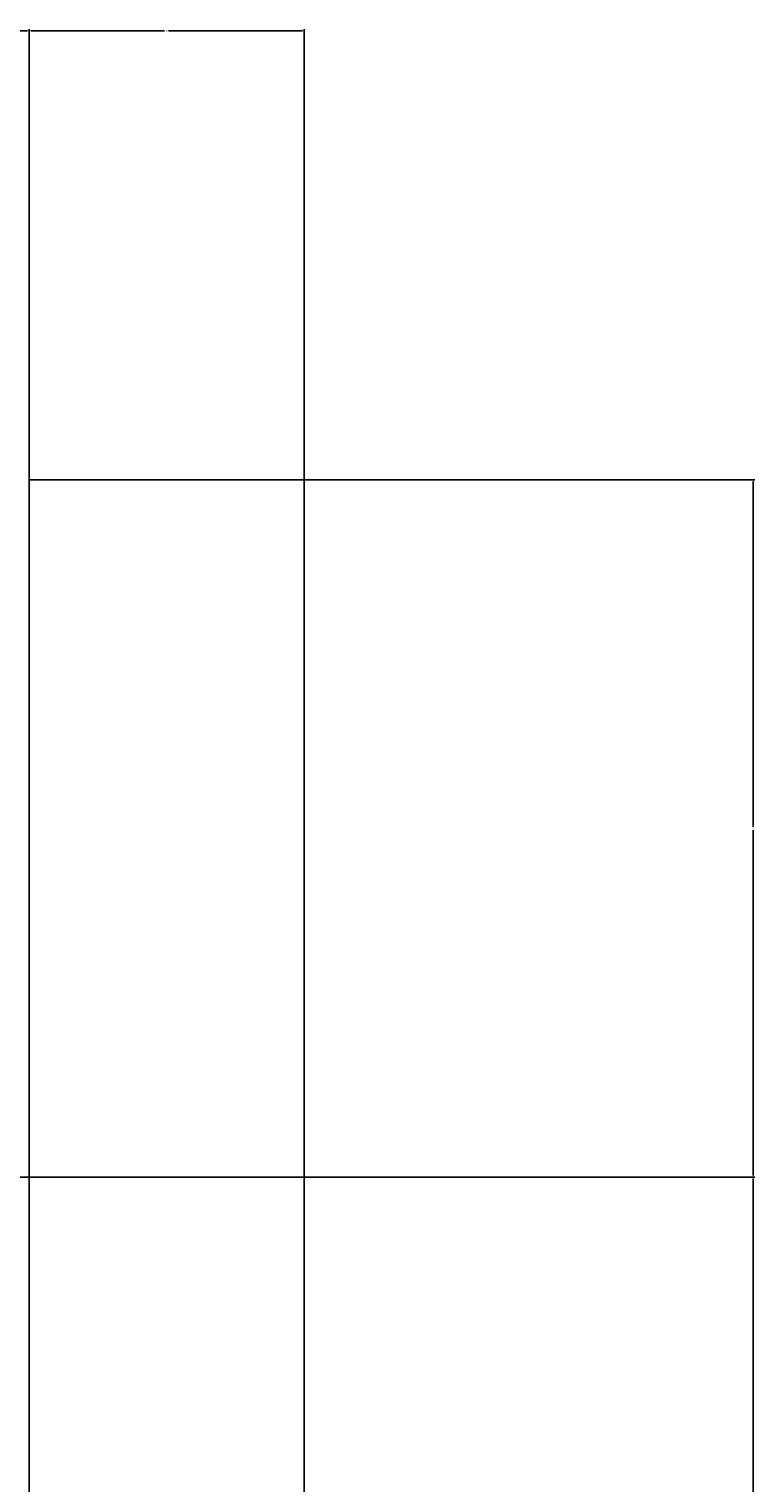
# Model space of a CAD drawing. Units: inches. Extents: x 3731 to 4318, y 1310 to 2388.
# Tile 57 of 57: x 4239 to 4318, y 2229 to 2388. Entities that reach past the tile are written whole.
import ezdxf

# ---------------------------------------------------------------- set-up
doc = ezdxf.new("R2010")
doc.units = ezdxf.units.IN
doc.layers.add('A-ANNO-DIMS', color=2, linetype='Continuous', lineweight=18)
doc.styles.get("Standard").update_dxf_attribs({"font": 'arial.ttf'})
doc.dimstyles.get("Standard").update_dxf_attribs({"dimtxt": 0.18, "dimasz": 0.18, "dimexe": 0.18, "dimexo": 0.0625, "dimgap": 0.09, "dimtad": 0, "dimtih": 1, "dimtoh": 1, "dimdec": 4, "dimzin": 0, "dimdsep": 46, "dimtxsty": 'Standard', "dimcen": 0.09, "dimadec": 0, "dimazin": 0, "dimtfac": 1, "dimtdec": 4, "dimtofl": 0, "dimtmove": 0, "dimatfit": 3, "dimfxl": 1, "dimtolj": 1, "dimtzin": 0, "dimarcsym": 0})

# ---------------------------------------------------------------- blocks, each defined once
blk = doc.blocks.new('*D36')
at = {"layer": 'A-ANNO-DIMS', "color": 0, "lineweight": -2, "transparency": 16777216}
for p, q in [((4103.21, 2338.44), (4103.21, 2387.51)), ((4103.39, 2387.33), (4170.93, 2387.33)), ((4239.03, 2387.33), (4171.49, 2387.33)), ((4239.21, 2338.44), (4239.21, 2387.51))]:
    blk.add_line(p, q, dxfattribs=at)
at = {"layer": 'A-ANNO-DIMS', "color": 0, "transparency": 16777216}
for points in [[(4103.39, 2387.36), (4103.39, 2387.3), (4103.21, 2387.33)], [(4239.03, 2387.36), (4239.03, 2387.3), (4239.21, 2387.33)]]:
    blk.add_solid(points, dxfattribs=at)
at = {"layer": 'Defpoints', "color": 0, "transparency": 16777216}
for p in [(4239.21, 2387.33), (4103.21, 2338.38), (4239.21, 2338.38)]:
    blk.add_point(p, dxfattribs=at)
at = {"layer": 'A-ANNO-DIMS', "color": 0, "transparency": 16777216, "insert": (4171.21, 2387.33), "char_height": 0.18, "attachment_point": 5}
blk.add_mtext('\\A1;136', dxfattribs=at)
blk = doc.blocks.new('*D37')
at = {"layer": 'A-ANNO-DIMS', "color": 0, "lineweight": -2, "transparency": 16777216}
for p, q in [((4239.27, 2338.38), (4318.34, 2338.38)), ((4318.16, 2338.2), (4318.16, 2300.56)), ((4318.16, 2262.56), (4318.16, 2300.2)), ((4103.27, 2262.38), (4318.34, 2262.38))]:
    blk.add_line(p, q, dxfattribs=at)
at = {"layer": 'A-ANNO-DIMS', "color": 0, "transparency": 16777216}
for points in [[(4318.13, 2338.2), (4318.19, 2338.2), (4318.16, 2338.38)], [(4318.13, 2262.56), (4318.19, 2262.56), (4318.16, 2262.38)]]:
    blk.add_solid(points, dxfattribs=at)
at = {"layer": 'Defpoints', "color": 0, "transparency": 16777216}
for p in [(4239.21, 2338.38), (4318.16, 2338.38), (4103.21, 2262.38)]:
    blk.add_point(p, dxfattribs=at)
at = {"layer": 'A-ANNO-DIMS', "color": 0, "transparency": 16777216, "insert": (4318.16, 2300.38), "char_height": 0.18, "attachment_point": 5}
blk.add_mtext('\\A1;76', dxfattribs=at)
blk = doc.blocks.new('*D38')
at = {"layer": 'A-ANNO-DIMS', "color": 0, "lineweight": -2, "transparency": 16777216}
for p, q in [((4103.27, 2262.38), (4318.34, 2262.38)), ((4318.16, 2262.2), (4318.16, 2103.06)), ((4318.16, 1943.56), (4318.16, 2102.7)), ((4234.27, 1943.38), (4318.34, 1943.38))]:
    blk.add_line(p, q, dxfattribs=at)
at = {"layer": 'A-ANNO-DIMS', "color": 0, "transparency": 16777216}
for points in [[(4318.13, 2262.2), (4318.19, 2262.2), (4318.16, 2262.38)], [(4318.13, 1943.56), (4318.19, 1943.56), (4318.16, 1943.38)]]:
    blk.add_solid(points, dxfattribs=at)
at = {"layer": 'Defpoints', "color": 0, "transparency": 16777216}
for p in [(4103.21, 2262.38), (4318.16, 2262.38), (4234.21, 1943.38)]:
    blk.add_point(p, dxfattribs=at)
at = {"layer": 'A-ANNO-DIMS', "color": 0, "transparency": 16777216, "insert": (4318.16, 2102.88), "char_height": 0.18, "attachment_point": 5}
blk.add_mtext('\\A1;319', dxfattribs=at)
blk = doc.blocks.new('*D51')
at = {"layer": 'A-ANNO-DIMS', "color": 0, "lineweight": -2, "transparency": 16777216}
for p, q in [((4239.21, 1708.44), (4239.21, 2387.51)), ((4239.39, 2387.33), (4253.99, 2387.33)), ((4269.03, 2387.33), (4254.43, 2387.33)), ((4269.21, 1708.44), (4269.21, 2387.51))]:
    blk.add_line(p, q, dxfattribs=at)
at = {"layer": 'A-ANNO-DIMS', "color": 0, "transparency": 16777216}
for points in [[(4239.39, 2387.36), (4239.39, 2387.3), (4239.21, 2387.33)], [(4269.03, 2387.36), (4269.03, 2387.3), (4269.21, 2387.33)]]:
    blk.add_solid(points, dxfattribs=at)
at = {"layer": 'Defpoints', "color": 0, "transparency": 16777216}
for p in [(4269.21, 2387.33), (4239.21, 1708.38), (4269.21, 1708.38)]:
    blk.add_point(p, dxfattribs=at)
at = {"layer": 'A-ANNO-DIMS', "color": 0, "transparency": 16777216, "insert": (4254.21, 2387.33), "char_height": 0.18, "attachment_point": 5}
blk.add_mtext('\\A1;30', dxfattribs=at)

msp = doc.modelspace()

# ---------------------------------------------------------------- dimensions: what is measured, and where the dimension line sits
at = {"layer": 'A-ANNO-DIMS'}
for base, p1, p2, picture, middle in [((4239.21, 2387.33), (4103.21, 2338.38), (4239.21, 2338.38), '*D36', (4171.21, 2387.33)), ((4269.21, 2387.33), (4239.21, 1708.38), (4269.21, 1708.38), '*D51', (4254.21, 2387.33))]:
    dim = msp.add_linear_dim(base=base, p1=p1, p2=p2, dimstyle='Standard', override={"dimdec": 0, "dimlfac": 1, "dimrnd": 0, "dimzin": 0, "dimdsep": 46, "dimlunit": 2}, dxfattribs=at)
    dim.commit()
    dim.dimension.update_dxf_attribs({"geometry": picture, "text_midpoint": middle})
for base, p1, p2, picture, middle in [((4318.16, 2338.38), (4103.21, 2262.38), (4239.21, 2338.38), '*D37', (4318.16, 2300.38)), ((4318.16, 2262.38), (4234.21, 1943.38), (4103.21, 2262.38), '*D38', (4318.16, 2102.88))]:
    dim = msp.add_linear_dim(base=base, p1=p1, p2=p2, angle=90, dimstyle='Standard', override={"dimdec": 0, "dimlfac": 1, "dimrnd": 0, "dimzin": 0, "dimdsep": 46, "dimlunit": 2}, dxfattribs=at)
    dim.commit()
    dim.dimension.update_dxf_attribs({"geometry": picture, "text_midpoint": middle})

doc.saveas('drawing.dxf')
